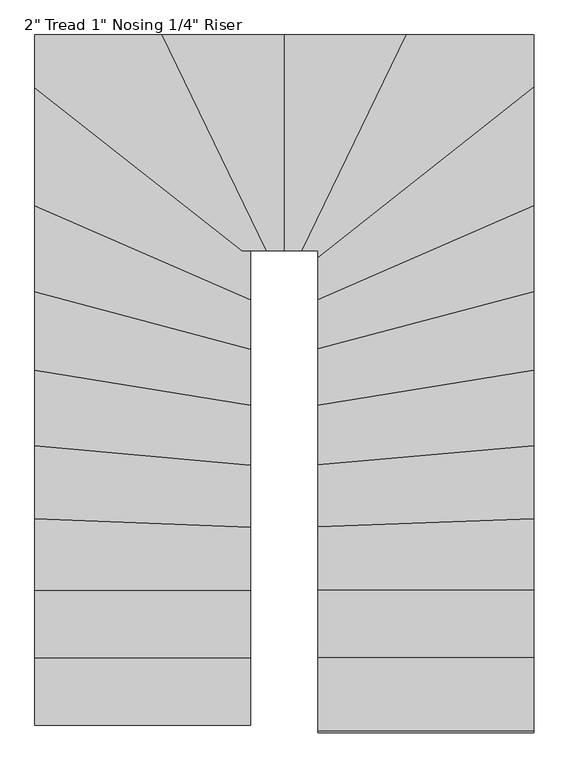
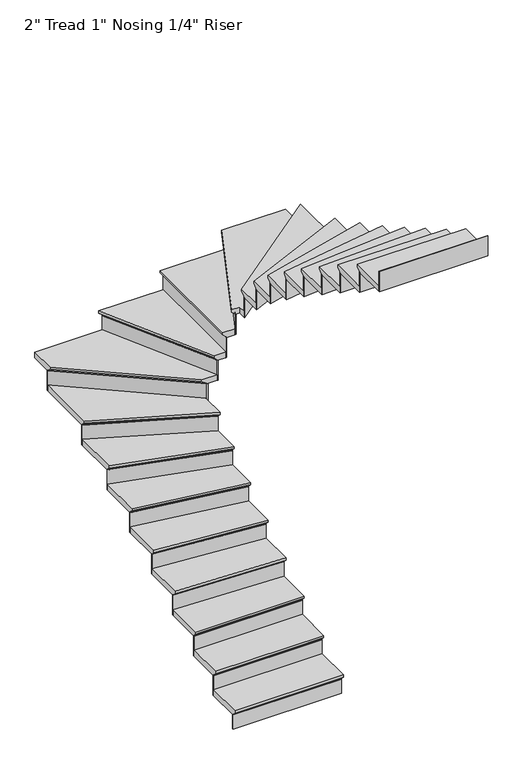
"""IFC4 building model written with IfcOpenShell, lengths in millimetres: stair flight geometry."""

from ifc_helpers import new_model, si_unit, origin, place, context, project, spatial, faceted_brep, source, transform, mapped, element, save


def stair_flight_aac49ba0(model_context):
    return source(origin(), model_context, "Body", "Brep", [
        faceted_brep([(-5047.1987704, -4554.2130548, 36731.1214286), (-5047.1987704, -4554.2130548, 36750.1714286), (-5940.8822214, -4554.2130548, 36750.1714286), (-5940.8822214, -4554.2130548, 36731.1214286), (-5047.1987704, -4528.8130548, 36705.7214286), (-5940.8822214, -4528.8130548, 36705.7214286), (-5047.1987704, -4249.4130548, 36750.1714286), (-5940.8822214, -4249.4130548, 36750.1714286), (-5940.8822214, -4528.8130548, 36699.3714286), (-5940.8822214, -4249.4130548, 36699.3714286), (-5047.1987704, -4249.4130548, 36699.3714286), (-5047.1987704, -4528.8130548, 36699.3714286)], [[[0, 1, 2, 3]], [[4, 0, 3, 5]], [[2, 1, 6, 7]], [[8, 9, 10, 11]], [[2, 7, 9, 8, 5, 3]], [[8, 11, 4, 5]], [[6, 1, 0, 4, 11, 10]], [[7, 6, 10, 9]]]),
        faceted_brep([(-5047.1987704, -4528.8130548, 36699.3714286), (-5047.1987704, -4528.8130548, 36576.0), (-5047.1987704, -4522.4630548, 36576.0), (-5047.1987704, -4522.4630548, 36699.3714286), (-5940.8822214, -4528.8130548, 36699.3714286), (-5940.8822214, -4522.4630548, 36699.3714286), (-5940.8822214, -4522.4630548, 36576.0), (-5940.8822214, -4528.8130548, 36576.0)], [[[0, 1, 2, 3]], [[4, 5, 6, 7]], [[1, 0, 4, 7]], [[2, 1, 7, 6]], [[3, 2, 6, 5]], [[0, 3, 5, 4]]]),
        faceted_brep([(-5047.1987704, -4249.4130548, 36873.5428571), (-5047.1987704, -4249.4130548, 36699.3714286), (-5047.1987704, -4243.0630548, 36699.3714286), (-5047.1987704, -4243.0630548, 36873.5428571), (-5940.8822214, -4249.4130548, 36873.5428571), (-5940.8822214, -4243.0630548, 36873.5428571), (-5940.8822214, -4243.0630548, 36699.3714286), (-5940.8822214, -4249.4130548, 36699.3714286)], [[[0, 1, 2, 3]], [[4, 5, 6, 7]], [[1, 0, 4, 7]], [[2, 1, 7, 6]], [[3, 2, 6, 5]], [[0, 3, 5, 4]]]),
        faceted_brep([(-5940.8822214, -4274.8130548, 36924.3428571), (-5047.1987704, -4274.8130548, 36924.3428571), (-5047.1987704, -3970.0130548, 36924.3428571), (-5940.8822214, -3970.0130548, 36924.3428571), (-5940.8822214, -4249.4130548, 36873.5428571), (-5940.8822214, -3970.0130548, 36873.5428571), (-5047.1987704, -3970.0130548, 36873.5428571), (-5047.1987704, -4249.4130548, 36873.5428571), (-5940.8822214, -4249.4130548, 36879.8928571), (-5940.8822214, -4274.8130548, 36905.2928571), (-5047.1987704, -4249.4130548, 36879.8928571), (-5047.1987704, -4274.8130548, 36905.2928571)], [[[0, 1, 2, 3]], [[4, 5, 6, 7]], [[0, 3, 5, 4, 8, 9]], [[4, 7, 10, 8]], [[2, 1, 11, 10, 7, 6]], [[3, 2, 6, 5]], [[11, 1, 0, 9]], [[10, 11, 9, 8]]]),
        faceted_brep([(-5047.1987704, -3970.0130548, 37047.7142857), (-5047.1987704, -3970.0130548, 36873.5428571), (-5047.1987704, -3963.6630548, 36873.5428571), (-5047.1987704, -3963.6630548, 37047.7142857), (-5940.8822214, -3970.0130548, 37047.7142857), (-5940.8822214, -3963.6630548, 37047.7142857), (-5940.8822214, -3963.6630548, 36873.5428571), (-5940.8822214, -3970.0130548, 36873.5428571)], [[[0, 1, 2, 3]], [[4, 5, 6, 7]], [[1, 0, 4, 7]], [[2, 1, 7, 6]], [[3, 2, 6, 5]], [[0, 3, 5, 4]]]),
        faceted_brep([(-5940.8822214, -3995.4130548, 37098.5142857), (-5047.1987704, -3995.4130548, 37098.5142857), (-5047.1987704, -3707.9036879, 37098.5142857), (-5940.8822214, -3673.2843203, 37098.5142857), (-5940.8822214, -3970.0130548, 37047.7142857), (-5940.8822214, -3673.2843203, 37047.7142857), (-5047.1987704, -3707.9036879, 37047.7142857), (-5047.1987704, -3970.0130548, 37047.7142857), (-5940.8822214, -3970.0130548, 37054.0642857), (-5940.8822214, -3995.4130548, 37079.4642857), (-5047.1987704, -3970.0130548, 37054.0642857), (-5047.1987704, -3995.4130548, 37079.4642857)], [[[0, 1, 2, 3]], [[4, 5, 6, 7]], [[0, 3, 5, 4, 8, 9]], [[4, 7, 10, 8]], [[2, 1, 11, 10, 7, 6]], [[3, 2, 6, 5]], [[11, 1, 0, 9]], [[10, 11, 9, 8]]]),
        faceted_brep([(-5047.1987704, -3707.9036879, 37221.8857143), (-5047.1987704, -3707.9036879, 37047.7142857), (-5047.1987704, -3701.5489252, 37047.7142857), (-5047.1987704, -3701.5489252, 37221.8857143), (-5940.8822214, -3673.2843203, 37221.8857143), (-5940.8822214, -3666.9295576, 37221.8857143), (-5940.8822214, -3666.9295576, 37047.7142857), (-5940.8822214, -3673.2843203, 37047.7142857)], [[[0, 1, 2, 3]], [[4, 5, 6, 7]], [[1, 0, 4, 7]], [[2, 1, 7, 6]], [[3, 2, 6, 5]], [[0, 3, 5, 4]]]),
        faceted_brep([(-5940.8822214, -3698.703371, 37272.6857143), (-5047.1987704, -3733.3227386, 37272.6857143), (-5047.1987704, -3451.3234819, 37272.6857143), (-5940.8822214, -3370.89733, 37272.6857143), (-5940.8822214, -3673.2843203, 37221.8857143), (-5940.8822214, -3370.89733, 37221.8857143), (-5047.1987704, -3451.3234819, 37221.8857143), (-5047.1987704, -3707.9036879, 37221.8857143), (-5940.8822214, -3673.2843203, 37228.2357143), (-5940.8822214, -3698.703371, 37253.6357143), (-5047.1987704, -3707.9036879, 37228.2357143), (-5047.1987704, -3733.3227386, 37253.6357143)], [[[0, 1, 2, 3]], [[4, 5, 6, 7]], [[0, 3, 5, 4, 8, 9]], [[4, 7, 10, 8]], [[2, 1, 11, 10, 7, 6]], [[3, 2, 6, 5]], [[11, 1, 0, 9]], [[10, 11, 9, 8]]]),
        faceted_brep([(-5047.1987704, -3451.3234819, 37396.0571429), (-5047.1987704, -3451.3234819, 37221.8857143), (-5047.1987704, -3444.9478197, 37221.8857143), (-5047.1987704, -3444.9478197, 37396.0571429), (-5940.8822214, -3370.89733, 37396.0571429), (-5940.8822214, -3364.5216678, 37396.0571429), (-5940.8822214, -3364.5216678, 37221.8857143), (-5940.8822214, -3370.89733, 37221.8857143)], [[[0, 1, 2, 3]], [[4, 5, 6, 7]], [[1, 0, 4, 7]], [[2, 1, 7, 6]], [[3, 2, 6, 5]], [[0, 3, 5, 4]]]),
        faceted_brep([(-5940.8822214, -3396.3999789, 37446.8571429), (-5047.1987704, -3476.8261308, 37446.8571429), (-5047.1987704, -3203.4301079, 37446.8571429), (-5940.8822214, -3059.5417727, 37446.8571429), (-5940.8822214, -3370.89733, 37396.0571429), (-5940.8822214, -3059.5417727, 37396.0571429), (-5047.1987704, -3203.4301079, 37396.0571429), (-5047.1987704, -3451.3234819, 37396.0571429), (-5940.8822214, -3370.89733, 37402.4071429), (-5940.8822214, -3396.3999789, 37427.8071429), (-5047.1987704, -3451.3234819, 37402.4071429), (-5047.1987704, -3476.8261308, 37427.8071429)], [[[0, 1, 2, 3]], [[4, 5, 6, 7]], [[0, 3, 5, 4, 8, 9]], [[4, 7, 10, 8]], [[2, 1, 11, 10, 7, 6]], [[3, 2, 6, 5]], [[11, 1, 0, 9]], [[10, 11, 9, 8]]]),
        faceted_brep([(-5047.1987704, -3203.4301079, 37570.2285714), (-5047.1987704, -3203.4301079, 37396.0571429), (-5047.1987704, -3196.9983292, 37396.0571429), (-5047.1987704, -3196.9983292, 37570.2285714), (-5940.8822214, -3059.5417727, 37570.2285714), (-5940.8822214, -3053.109994, 37570.2285714), (-5940.8822214, -3053.109994, 37396.0571429), (-5940.8822214, -3059.5417727, 37396.0571429)], [[[0, 1, 2, 3]], [[4, 5, 6, 7]], [[1, 0, 4, 7]], [[2, 1, 7, 6]], [[3, 2, 6, 5]], [[0, 3, 5, 4]]]),
        faceted_brep([(-5940.8822214, -3085.2688872, 37621.0285714), (-5047.1987704, -3229.1572224, 37621.0285714), (-5047.1987704, -2970.3553609, 37621.0285714), (-5940.8822214, -2732.7052783, 37621.0285714), (-5940.8822214, -3059.5417727, 37570.2285714), (-5940.8822214, -2732.7052783, 37570.2285714), (-5047.1987704, -2970.3553609, 37570.2285714), (-5047.1987704, -3203.4301079, 37570.2285714), (-5940.8822214, -3059.5417727, 37576.5785714), (-5940.8822214, -3085.2688872, 37601.9785714), (-5047.1987704, -3203.4301079, 37576.5785714), (-5047.1987704, -3229.1572224, 37601.9785714)], [[[0, 1, 2, 3]], [[4, 5, 6, 7]], [[0, 3, 5, 4, 8, 9]], [[4, 7, 10, 8]], [[2, 1, 11, 10, 7, 6]], [[3, 2, 6, 5]], [[11, 1, 0, 9]], [[10, 11, 9, 8]]]),
        faceted_brep([(-5047.1987704, -2970.3553609, 37744.4), (-5047.1987704, -2970.3553609, 37570.2285714), (-5047.1987704, -2963.7846771, 37570.2285714), (-5047.1987704, -2963.7846771, 37744.4), (-5940.8822214, -2732.7052783, 37744.4), (-5940.8822214, -2726.1345945, 37744.4), (-5940.8822214, -2726.1345945, 37570.2285714), (-5940.8822214, -2732.7052783, 37570.2285714)], [[[0, 1, 2, 3]], [[4, 5, 6, 7]], [[1, 0, 4, 7]], [[2, 1, 7, 6]], [[3, 2, 6, 5]], [[0, 3, 5, 4]]]),
        faceted_brep([(-5940.8822214, -2758.9880136, 37795.2), (-5047.1987704, -2996.6380961, 37795.2), (-5047.1987704, -2765.8050203, 37795.2), (-5940.8822214, -2375.5896532, 37795.2), (-5940.8822214, -2732.7052783, 37744.4), (-5940.8822214, -2375.5896532, 37744.4), (-5047.1987704, -2765.8050203, 37744.4), (-5047.1987704, -2970.3553609, 37744.4), (-5940.8822214, -2732.7052783, 37750.75), (-5940.8822214, -2758.9880136, 37776.15), (-5047.1987704, -2970.3553609, 37750.75), (-5047.1987704, -2996.6380961, 37776.15)], [[[0, 1, 2, 3]], [[4, 5, 6, 7]], [[0, 3, 5, 4, 8, 9]], [[4, 7, 10, 8]], [[2, 1, 11, 10, 7, 6]], [[3, 2, 6, 5]], [[11, 1, 0, 9]], [[10, 11, 9, 8]]]),
        faceted_brep([(-5047.1987704, -2765.8050203, 37918.5714286), (-5047.1987704, -2765.8050203, 37744.4), (-5047.1987704, -2758.8760908, 37744.4), (-5047.1987704, -2758.8760908, 37918.5714286), (-5940.8822214, -2375.5896532, 37918.5714286), (-5940.8822214, -2368.6607237, 37918.5714286), (-5940.8822214, -2368.6607237, 37744.4), (-5940.8822214, -2375.5896532, 37744.4)], [[[0, 1, 2, 3]], [[4, 5, 6, 7]], [[1, 0, 4, 7]], [[2, 1, 7, 6]], [[3, 2, 6, 5]], [[0, 3, 5, 4]]]),
        faceted_brep([(-5940.8822214, -2403.3053713, 37969.3714286), (-5047.1987704, -2793.5207384, 37969.3714286), (-5047.1987704, -2590.8424524, 37969.3714286), (-5040.8038639, -2590.8424524, 37969.3714286), (-5940.8822214, -1882.1944717, 37969.3714286), (-5940.8822214, -2375.5896532, 37918.5714286), (-5940.8822214, -1882.1944717, 37918.5714286), (-5040.8038639, -2590.8424524, 37918.5714286), (-5047.1987704, -2590.8424524, 37918.5714286), (-5047.1987704, -2765.8050203, 37918.5714286), (-5940.8822214, -2375.5896532, 37924.9214286), (-5940.8822214, -2403.3053713, 37950.3214286), (-5047.1987704, -2765.8050203, 37924.9214286), (-5047.1987704, -2793.5207384, 37950.3214286)], [[[0, 1, 2, 3, 4]], [[5, 6, 7, 8, 9]], [[0, 4, 6, 5, 10, 11]], [[5, 9, 12, 10]], [[2, 1, 13, 12, 9, 8]], [[4, 3, 7, 6]], [[13, 1, 0, 11]], [[12, 13, 11, 10]], [[3, 2, 8, 7]]]),
        faceted_brep([(-5040.8038639, -2590.8424524, 38092.7428571), (-5040.8038639, -2590.8424524, 37918.5714286), (-5030.5387554, -2590.8424524, 37918.5714286), (-5030.5387554, -2590.8424524, 38092.7428571), (-5940.8822214, -1882.1944717, 38092.7428571), (-5940.8822214, -1874.1125661, 38092.7428571), (-5940.8822214, -1874.1125661, 37918.5714286), (-5940.8822214, -1882.1944717, 37918.5714286)], [[[0, 1, 2, 3]], [[4, 5, 6, 7]], [[1, 0, 4, 7]], [[2, 1, 7, 6]], [[3, 2, 6, 5]], [[0, 3, 5, 4]]]),
        faceted_brep([(-5384.6489457, -1697.1590014, 38143.5428571), (-5940.8822214, -1697.1590014, 38143.5428571), (-5940.8822214, -1914.5220945, 38143.5428571), (-5081.8642978, -2590.8424524, 38143.5428571), (-4952.3566185, -2590.8424524, 38143.5428571), (-5940.8822214, -1697.1590014, 38092.7428571), (-5384.6489457, -1697.1590014, 38092.7428571), (-4952.3566185, -2590.8424524, 38092.7428571), (-5040.8038639, -2590.8424524, 38092.7428571), (-5940.8822214, -1882.1944717, 38092.7428571), (-5940.8822214, -1882.1944717, 38099.0928571), (-5940.8822214, -1914.5220945, 38124.4928571), (-5040.8038639, -2590.8424524, 38099.0928571), (-5081.8642978, -2590.8424524, 38124.4928571)], [[[0, 1, 2, 3, 4]], [[5, 6, 7, 8, 9]], [[1, 0, 6, 5]], [[2, 1, 5, 9, 10, 11]], [[9, 8, 12, 10]], [[4, 3, 13, 12, 8, 7]], [[0, 4, 7, 6]], [[13, 3, 2, 11]], [[12, 13, 11, 10]]]),
        faceted_brep([(-4952.3566185, -2590.8424524, 38266.9142857), (-4952.3566185, -2590.8424524, 38092.7428571), (-4945.3027294, -2590.8424524, 38092.7428571), (-4945.3027294, -2590.8424524, 38266.9142857), (-5384.6489457, -1697.1590014, 38266.9142857), (-5377.5950566, -1697.1590014, 38266.9142857), (-5377.5950566, -1697.1590014, 38092.7428571), (-5384.6489457, -1697.1590014, 38092.7428571)], [[[0, 1, 2, 3]], [[4, 5, 6, 7]], [[1, 0, 4, 7]], [[2, 1, 7, 6]], [[3, 2, 6, 5]], [[0, 3, 5, 4]]]),
        faceted_brep([(-5412.8645022, -1697.1590014, 38317.7142857), (-4980.5721749, -2590.8424524, 38317.7142857), (-4882.0987704, -2590.8424524, 38317.7142857), (-4882.0987706, -1697.1590014, 38317.7142857), (-5384.6489457, -1697.1590014, 38266.9142857), (-4882.0987706, -1697.1590014, 38266.9142857), (-4882.0987704, -2590.8424524, 38266.9142857), (-4952.3566185, -2590.8424524, 38266.9142857), (-5384.6489457, -1697.1590014, 38273.2642857), (-5412.8645022, -1697.1590014, 38298.6642857), (-4952.3566185, -2590.8424524, 38273.2642857), (-4980.5721749, -2590.8424524, 38298.6642857)], [[[0, 1, 2, 3]], [[4, 5, 6, 7]], [[0, 3, 5, 4, 8, 9]], [[4, 7, 10, 8]], [[3, 2, 6, 5]], [[11, 1, 0, 9]], [[10, 11, 9, 8]], [[2, 1, 11, 10, 7, 6]]]),
        faceted_brep([(-4882.0987704, -2590.8424524, 38441.0857143), (-4882.0987704, -2590.8424524, 38266.9142857), (-4875.7487704, -2590.8424524, 38266.9142857), (-4875.7487704, -2590.8424524, 38441.0857143), (-4882.0987706, -1697.1590014, 38441.0857143), (-4875.7487706, -1697.1590014, 38441.0857143), (-4875.7487706, -1697.1590014, 38266.9142857), (-4882.0987706, -1697.1590014, 38266.9142857)], [[[0, 1, 2, 3]], [[4, 5, 6, 7]], [[1, 0, 4, 7]], [[2, 1, 7, 6]], [[3, 2, 6, 5]], [[0, 3, 5, 4]]]),
        faceted_brep([(-4907.4987706, -1697.1590014, 38491.8857143), (-4907.4987704, -2590.8424524, 38491.8857143), (-4806.2098095, -2590.8424524, 38491.8857143), (-4373.9174828, -1697.1590014, 38491.8857143), (-4882.0987706, -1697.1590014, 38441.0857143), (-4373.9174828, -1697.1590014, 38441.0857143), (-4806.2098095, -2590.8424524, 38441.0857143), (-4882.0987704, -2590.8424524, 38441.0857143), (-4882.0987706, -1697.1590014, 38447.4357143), (-4907.4987706, -1697.1590014, 38472.8357143), (-4882.0987704, -2590.8424524, 38447.4357143), (-4907.4987704, -2590.8424524, 38472.8357143)], [[[0, 1, 2, 3]], [[4, 5, 6, 7]], [[0, 3, 5, 4, 8, 9]], [[4, 7, 10, 8]], [[2, 1, 11, 10, 7, 6]], [[3, 2, 6, 5]], [[11, 1, 0, 9]], [[10, 11, 9, 8]]]),
        faceted_brep([(-4806.2098095, -2590.8424524, 38615.2571429), (-4806.2098095, -2590.8424524, 38441.0857143), (-4799.1559204, -2590.8424524, 38441.0857143), (-4799.1559204, -2590.8424524, 38615.2571429), (-4373.9174828, -1697.1590014, 38615.2571429), (-4366.8635937, -1697.1590014, 38615.2571429), (-4366.8635937, -1697.1590014, 38441.0857143), (-4373.9174828, -1697.1590014, 38441.0857143)], [[[0, 1, 2, 3]], [[4, 5, 6, 7]], [[1, 0, 4, 7]], [[2, 1, 7, 6]], [[3, 2, 6, 5]], [[0, 3, 5, 4]]]),
        faceted_brep([(-3874.1153195, -1946.8497166, 38666.0571429), (-3874.1153195, -1697.1590014, 38666.0571429), (-4402.1330392, -1697.1590014, 38666.0571429), (-4834.4253659, -2590.8424524, 38666.0571429), (-4767.7987704, -2590.8424524, 38666.0571429), (-4767.7987704, -2650.4628721, 38666.0571429), (-3874.1153195, -1697.1590014, 38615.2571429), (-3874.1153195, -1946.8497166, 38615.2571429), (-4767.7987704, -2650.4628721, 38615.2571429), (-4767.7987704, -2590.8424524, 38615.2571429), (-4806.2098095, -2590.8424524, 38615.2571429), (-4373.9174828, -1697.1590014, 38615.2571429), (-4806.2098095, -2590.8424524, 38621.6071429), (-4373.9174828, -1697.1590014, 38621.6071429), (-4834.4253659, -2590.8424524, 38647.0071429), (-4402.1330392, -1697.1590014, 38647.0071429)], [[[0, 1, 2, 3, 4, 5]], [[6, 7, 8, 9, 10, 11]], [[1, 0, 7, 6]], [[11, 10, 12, 13]], [[4, 3, 14, 12, 10, 9]], [[5, 4, 9, 8]], [[0, 5, 8, 7]], [[14, 3, 2, 15]], [[12, 14, 15, 13]], [[2, 1, 6, 11, 13, 15]]]),
        faceted_brep([(-4767.7987704, -2650.4628721, 38789.4285714), (-4767.7987704, -2650.4628721, 38615.2571429), (-4767.7987704, -2658.5447778, 38615.2571429), (-4767.7987704, -2658.5447778, 38789.4285714), (-3874.1153195, -1946.8497166, 38789.4285714), (-3874.1153195, -1954.9316222, 38789.4285714), (-3874.1153195, -1954.9316222, 38615.2571429), (-3874.1153195, -1946.8497166, 38615.2571429)], [[[0, 1, 2, 3]], [[4, 5, 6, 7]], [[1, 0, 4, 7]], [[2, 1, 7, 6]], [[3, 2, 6, 5]], [[0, 3, 5, 4]]]),
        faceted_brep([(-3874.1153195, -1914.5220938, 38840.2285714), (-4767.7987704, -2618.1352494, 38840.2285714), (-4767.7987704, -2821.2364563, 38840.2285714), (-3874.1153195, -2431.0210889, 38840.2285714), (-3874.1153195, -1946.8497166, 38789.4285714), (-3874.1153195, -2431.0210889, 38789.4285714), (-4767.7987704, -2821.2364563, 38789.4285714), (-4767.7987704, -2650.4628721, 38789.4285714), (-3874.1153195, -1946.8497166, 38795.7785714), (-3874.1153195, -1914.5220938, 38821.1785714), (-4767.7987704, -2650.4628721, 38795.7785714), (-4767.7987704, -2618.1352494, 38821.1785714)], [[[0, 1, 2, 3]], [[4, 5, 6, 7]], [[0, 3, 5, 4, 8, 9]], [[4, 7, 10, 8]], [[2, 1, 11, 10, 7, 6]], [[3, 2, 6, 5]], [[11, 1, 0, 9]], [[10, 11, 9, 8]]]),
        faceted_brep([(-4767.7987704, -2821.2364563, 38963.6), (-4767.7987704, -2821.2364563, 38789.4285714), (-4767.7987704, -2828.1653858, 38789.4285714), (-4767.7987704, -2828.1653858, 38963.6), (-3874.1153195, -2431.0210889, 38963.6), (-3874.1153195, -2437.9500185, 38963.6), (-3874.1153195, -2437.9500185, 38789.4285714), (-3874.1153195, -2431.0210889, 38789.4285714)], [[[0, 1, 2, 3]], [[4, 5, 6, 7]], [[1, 0, 4, 7]], [[2, 1, 7, 6]], [[3, 2, 6, 5]], [[0, 3, 5, 4]]]),
        faceted_brep([(-3874.1153195, -2403.3053709, 39014.4), (-4767.7987704, -2793.5207382, 39014.4), (-4767.7987704, -3022.9208311, 39014.4), (-3874.1153195, -2785.2707484, 39014.4), (-3874.1153195, -2431.0210889, 38963.6), (-3874.1153195, -2785.2707484, 38963.6), (-4767.7987704, -3022.9208311, 38963.6), (-4767.7987704, -2821.2364563, 38963.6), (-3874.1153195, -2431.0210889, 38969.95), (-3874.1153195, -2403.3053709, 38995.35), (-4767.7987704, -2821.2364563, 38969.95), (-4767.7987704, -2793.5207382, 38995.35)], [[[0, 1, 2, 3]], [[4, 5, 6, 7]], [[0, 3, 5, 4, 8, 9]], [[4, 7, 10, 8]], [[2, 1, 11, 10, 7, 6]], [[3, 2, 6, 5]], [[11, 1, 0, 9]], [[10, 11, 9, 8]]]),
        faceted_brep([(-4767.7987704, -3022.9208311, 39137.7714286), (-4767.7987704, -3022.9208311, 38963.6), (-4767.7987704, -3029.4915149, 38963.6), (-4767.7987704, -3029.4915149, 39137.7714286), (-3874.1153195, -2785.2707484, 39137.7714286), (-3874.1153195, -2791.8414322, 39137.7714286), (-3874.1153195, -2791.8414322, 38963.6), (-3874.1153195, -2785.2707484, 38963.6)], [[[0, 1, 2, 3]], [[4, 5, 6, 7]], [[1, 0, 4, 7]], [[2, 1, 7, 6]], [[3, 2, 6, 5]], [[0, 3, 5, 4]]]),
        faceted_brep([(-3874.1153195, -2758.9880132, 39188.5714286), (-4767.7987704, -2996.6380959, 39188.5714286), (-4767.7987704, -3254.8843368, 39188.5714286), (-3874.1153195, -3110.9960015, 39188.5714286), (-3874.1153195, -2785.2707484, 39137.7714286), (-3874.1153195, -3110.9960015, 39137.7714286), (-4767.7987704, -3254.8843368, 39137.7714286), (-4767.7987704, -3022.9208311, 39137.7714286), (-3874.1153195, -2785.2707484, 39144.1214286), (-3874.1153195, -2758.9880132, 39169.5214286), (-4767.7987704, -3022.9208311, 39144.1214286), (-4767.7987704, -2996.6380959, 39169.5214286)], [[[0, 1, 2, 3]], [[4, 5, 6, 7]], [[0, 3, 5, 4, 8, 9]], [[4, 7, 10, 8]], [[2, 1, 11, 10, 7, 6]], [[3, 2, 6, 5]], [[11, 1, 0, 9]], [[10, 11, 9, 8]]]),
        faceted_brep([(-4767.7987704, -3254.8843368, 39311.9428571), (-4767.7987704, -3254.8843368, 39137.7714286), (-4767.7987704, -3261.3161154, 39137.7714286), (-4767.7987704, -3261.3161154, 39311.9428571), (-3874.1153195, -3110.9960015, 39311.9428571), (-3874.1153195, -3117.4277801, 39311.9428571), (-3874.1153195, -3117.4277801, 39137.7714286), (-3874.1153195, -3110.9960015, 39137.7714286)], [[[0, 1, 2, 3]], [[4, 5, 6, 7]], [[1, 0, 4, 7]], [[2, 1, 7, 6]], [[3, 2, 6, 5]], [[0, 3, 5, 4]]]),
        faceted_brep([(-3874.1153195, -3085.2688869, 39362.7428571), (-4767.7987704, -3229.1572222, 39362.7428571), (-4767.7987704, -3502.3287795, 39362.7428571), (-3874.1153195, -3421.9026274, 39362.7428571), (-3874.1153195, -3110.9960015, 39311.9428571), (-3874.1153195, -3421.9026274, 39311.9428571), (-4767.7987704, -3502.3287795, 39311.9428571), (-4767.7987704, -3254.8843368, 39311.9428571), (-3874.1153195, -3110.9960015, 39318.2928571), (-3874.1153195, -3085.2688869, 39343.6928571), (-4767.7987704, -3254.8843368, 39318.2928571), (-4767.7987704, -3229.1572222, 39343.6928571)], [[[0, 1, 2, 3]], [[4, 5, 6, 7]], [[0, 3, 5, 4, 8, 9]], [[4, 7, 10, 8]], [[2, 1, 11, 10, 7, 6]], [[3, 2, 6, 5]], [[11, 1, 0, 9]], [[10, 11, 9, 8]]]),
        faceted_brep([(-4767.7987704, -3502.3287795, 39486.1142857), (-4767.7987704, -3502.3287795, 39311.9428571), (-4767.7987704, -3508.7044417, 39311.9428571), (-4767.7987704, -3508.7044417, 39486.1142857), (-3874.1153195, -3421.9026274, 39486.1142857), (-3874.1153195, -3428.2782897, 39486.1142857), (-3874.1153195, -3428.2782897, 39311.9428571), (-3874.1153195, -3421.9026274, 39311.9428571)], [[[0, 1, 2, 3]], [[4, 5, 6, 7]], [[1, 0, 4, 7]], [[2, 1, 7, 6]], [[3, 2, 6, 5]], [[0, 3, 5, 4]]]),
        faceted_brep([(-3874.1153195, -3396.3999786, 39536.9142857), (-4767.7987704, -3476.8261306, 39536.9142857), (-4767.7987704, -3758.7417891, 39536.9142857), (-3874.1153195, -3724.1224215, 39536.9142857), (-3874.1153195, -3421.9026274, 39486.1142857), (-3874.1153195, -3724.1224215, 39486.1142857), (-4767.7987704, -3758.7417891, 39486.1142857), (-4767.7987704, -3502.3287795, 39486.1142857), (-3874.1153195, -3421.9026274, 39492.4642857), (-3874.1153195, -3396.3999786, 39517.8642857), (-4767.7987704, -3502.3287795, 39492.4642857), (-4767.7987704, -3476.8261306, 39517.8642857)], [[[0, 1, 2, 3]], [[4, 5, 6, 7]], [[0, 3, 5, 4, 8, 9]], [[4, 7, 10, 8]], [[2, 1, 11, 10, 7, 6]], [[3, 2, 6, 5]], [[11, 1, 0, 9]], [[10, 11, 9, 8]]]),
        faceted_brep([(-4767.7987704, -3758.7417891, 39660.2857143), (-4767.7987704, -3758.7417891, 39486.1142857), (-4767.7987704, -3765.0965518, 39486.1142857), (-4767.7987704, -3765.0965518, 39660.2857143), (-3874.1153195, -3724.1224215, 39660.2857143), (-3874.1153195, -3730.4771842, 39660.2857143), (-3874.1153195, -3730.4771842, 39486.1142857), (-3874.1153195, -3724.1224215, 39486.1142857)], [[[0, 1, 2, 3]], [[4, 5, 6, 7]], [[1, 0, 4, 7]], [[2, 1, 7, 6]], [[3, 2, 6, 5]], [[0, 3, 5, 4]]]),
        faceted_brep([(-3874.1153195, -3698.7033708, 39711.0857143), (-4767.7987704, -3733.3227384, 39711.0857143), (-4767.7987704, -4020.8130546, 39711.0857143), (-3874.1153195, -4020.8130546, 39711.0857143), (-3874.1153195, -3724.1224215, 39660.2857143), (-3874.1153195, -4020.8130546, 39660.2857143), (-4767.7987704, -4020.8130546, 39660.2857143), (-4767.7987704, -3758.7417891, 39660.2857143), (-3874.1153195, -3724.1224215, 39666.6357143), (-3874.1153195, -3698.7033708, 39692.0357143), (-4767.7987704, -3758.7417891, 39666.6357143), (-4767.7987704, -3733.3227384, 39692.0357143)], [[[0, 1, 2, 3]], [[4, 5, 6, 7]], [[0, 3, 5, 4, 8, 9]], [[4, 7, 10, 8]], [[2, 1, 11, 10, 7, 6]], [[3, 2, 6, 5]], [[11, 1, 0, 9]], [[10, 11, 9, 8]]]),
        faceted_brep([(-4767.7987704, -4020.8130546, 39834.4571429), (-4767.7987704, -4020.8130546, 39660.2857143), (-4767.7987704, -4027.1630546, 39660.2857143), (-4767.7987704, -4027.1630546, 39834.4571429), (-3874.1153195, -4020.8130546, 39834.4571429), (-3874.1153195, -4027.1630546, 39834.4571429), (-3874.1153195, -4027.1630546, 39660.2857143), (-3874.1153195, -4020.8130546, 39660.2857143)], [[[0, 1, 2, 3]], [[4, 5, 6, 7]], [[1, 0, 4, 7]], [[2, 1, 7, 6]], [[3, 2, 6, 5]], [[0, 3, 5, 4]]]),
        faceted_brep([(-3874.1153195, -3995.4130546, 39885.2571429), (-4767.7987704, -3995.4130546, 39885.2571429), (-4767.7987704, -4300.2130546, 39885.2571429), (-3874.1153195, -4300.2130546, 39885.2571429), (-3874.1153195, -4020.8130546, 39834.4571429), (-3874.1153195, -4300.2130546, 39834.4571429), (-4767.7987704, -4300.2130546, 39834.4571429), (-4767.7987704, -4020.8130546, 39834.4571429), (-3874.1153195, -4020.8130546, 39840.8071429), (-3874.1153195, -3995.4130546, 39866.2071429), (-4767.7987704, -4020.8130546, 39840.8071429), (-4767.7987704, -3995.4130546, 39866.2071429)], [[[0, 1, 2, 3]], [[4, 5, 6, 7]], [[0, 3, 5, 4, 8, 9]], [[4, 7, 10, 8]], [[2, 1, 11, 10, 7, 6]], [[3, 2, 6, 5]], [[11, 1, 0, 9]], [[10, 11, 9, 8]]]),
        faceted_brep([(-4767.7987704, -4300.2130546, 40008.6285714), (-4767.7987704, -4300.2130546, 39834.4571429), (-4767.7987704, -4306.5630546, 39834.4571429), (-4767.7987704, -4306.5630546, 40008.6285714), (-3874.1153195, -4300.2130546, 40008.6285714), (-3874.1153195, -4306.5630546, 40008.6285714), (-3874.1153195, -4306.5630546, 39834.4571429), (-3874.1153195, -4300.2130546, 39834.4571429)], [[[0, 1, 2, 3]], [[4, 5, 6, 7]], [[1, 0, 4, 7]], [[2, 1, 7, 6]], [[3, 2, 6, 5]], [[0, 3, 5, 4]]]),
        faceted_brep([(-4767.7987704, -4579.6130546, 40182.8), (-4767.7987704, -4579.6130546, 40008.6285714), (-4767.7987704, -4585.9630546, 40008.6285714), (-4767.7987704, -4585.9630546, 40182.8), (-3874.1153195, -4579.6130546, 40182.8), (-3874.1153195, -4585.9630546, 40182.8), (-3874.1153195, -4585.9630546, 40008.6285714), (-3874.1153195, -4579.6130546, 40008.6285714)], [[[0, 1, 2, 3]], [[4, 5, 6, 7]], [[1, 0, 4, 7]], [[2, 1, 7, 6]], [[3, 2, 6, 5]], [[0, 3, 5, 4]]]),
        faceted_brep([(-3874.1153195, -4274.8130546, 40059.4285714), (-4767.7987704, -4274.8130546, 40059.4285714), (-4767.7987704, -4579.6130546, 40059.4285714), (-3874.1153195, -4579.6130546, 40059.4285714), (-3874.1153195, -4300.2130546, 40008.6285714), (-3874.1153195, -4579.6130546, 40008.6285714), (-4767.7987704, -4579.6130546, 40008.6285714), (-4767.7987704, -4300.2130546, 40008.6285714), (-3874.1153195, -4300.2130546, 40014.9785714), (-3874.1153195, -4274.8130546, 40040.3785714), (-4767.7987704, -4300.2130546, 40014.9785714), (-4767.7987704, -4274.8130546, 40040.3785714)], [[[0, 1, 2, 3]], [[4, 5, 6, 7]], [[0, 3, 5, 4, 8, 9]], [[4, 7, 10, 8]], [[2, 1, 11, 10, 7, 6]], [[3, 2, 6, 5]], [[11, 1, 0, 9]], [[10, 11, 9, 8]]]),
    ])


if __name__ == "__main__":
    model = new_model("IFC4")
    model_context = context("Model", 3, world=origin())
    ifc_project = project(units=[si_unit("LENGTHUNIT", "METRE", prefix="MILLI")], contexts=[model_context])
    site = spatial("IfcSite", under=ifc_project)
    building = spatial("IfcBuilding", under=site)
    placement = place(None, origin())
    stair_flight_shape = stair_flight_aac49ba0(model_context)
    element("IfcStairFlight", 1, ObjectType="2\" Tread 1\" Nosing 1/4\" Riser", at=placement, inside=building, context=model_context, shape_type="MappedRepresentation", body=[
        mapped(stair_flight_shape, transform((0.0, 0.0, 0.0), x_axis=(1.0, 0.0, 0.0), y_axis=(0.0, 1.0, 0.0), z_axis=(0.0, 0.0, 1.0))),
    ])
    save(model, "model.ifc")

# Revit data of these elements
# Element 1 (IfcStairFlight, "2\" Tread 1\" Nosing 1/4\" Riser")
#   Materials on its faces: "Tile, Porcelain, 4in"
# Materials
#   "Tile, Porcelain, 4in": class "Generic", colour RGB 89 87 158, transparency 0, Description = "Porcelain tile, 4\", white", Cost = 0
